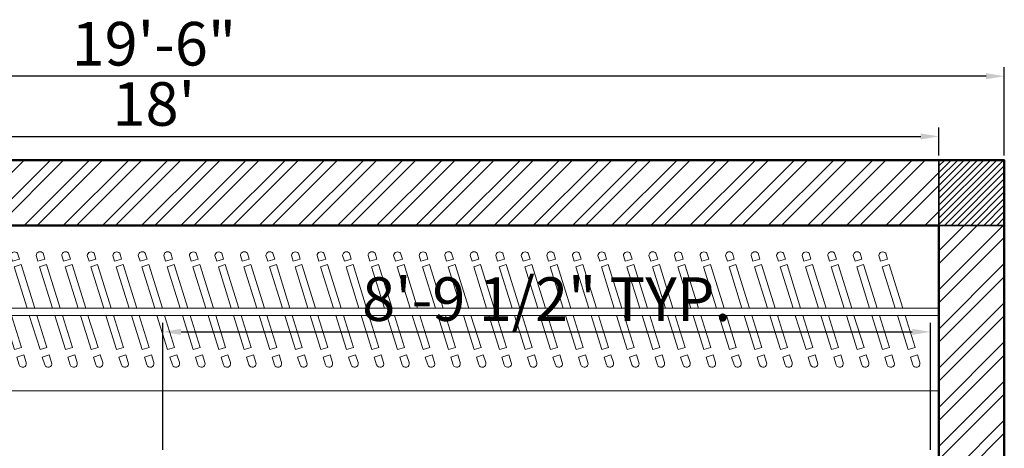
# Model space of a CAD drawing. Units: millimetres. Extents: x 20768 to 23556, y 50760 to 52704.
# Tile 23 of 36: x 20998 to 21133, y 52483 to 52542. Entities that reach past the tile are written whole.
import ezdxf

# ---------------------------------------------------------------- set-up
doc = ezdxf.new("R2010")
doc.units = ezdxf.units.MM
for name, color, linetype, lineweight in [('A-ANNO-DIMS', 2, 'Continuous', 18), ('A-FURN', 8, 'Continuous', 18), ('A-WALL', 7, 'Continuous', 50), ('A-WALL-PATT', 8, 'Continuous', 13), ('S-ANNO-DIMS', 2, 'Continuous', 18), ('S-COLS', 20, 'Continuous', 35)]:
    doc.layers.add(name, color=color, linetype=linetype, lineweight=lineweight)
doc.styles.get("Standard").update_dxf_attribs({"font": 'arial.ttf'})
doc.dimstyles.new('ISO-25', dxfattribs={"dimtxt": 6, "dimasz": 2.5, "dimexe": 1.25, "dimexo": 0.625, "dimtad": 1, "dimdec": 0, "dimlunit": 3, "dimtxsty": 'Standard', "dimcen": 2.5, "dimadec": 0, "dimazin": 0, "dimtfac": 1, "dimtdec": 0, "dimtmove": 0, "dimatfit": 3, "dimfxl": 1, "dimarcsym": 0})
pattern_1 = [(45, (-81.1113, 0), (-2.69407684, 2.69407684), []), (45, (-79.3152, 0), (-2.69407684, 2.69407684), [])]

# ---------------------------------------------------------------- blocks, each defined once
blk = doc.blocks.new('wb')
for p, q in [((21205.25, 52502.52), (21061.44, 52502.52)), ((21205.25, 52501.52), (21061.44, 52501.52))]:
    blk.add_line(p, q)
blk.add_lwpolyline([(21205.25, 52513.9), (21061.44, 52513.9), (21061.44, 52491.15), (21205.25, 52491.15)], close=True)
for points in [[(21064.45, 52510.07, 0.695903), (21063.5, 52509.77), (21063.75, 52508.98), (21064.7, 52509.27)], [(21067.97, 52510.07, 0.695903), (21067.01, 52509.77), (21067.26, 52508.98), (21068.21, 52509.27)], [(21071.48, 52510.07, 0.695903), (21070.52, 52509.77), (21070.77, 52508.98), (21071.73, 52509.27)], [(21074.99, 52510.07, 0.695903), (21074.04, 52509.77), (21074.28, 52508.98), (21075.24, 52509.27)], [(21078.5, 52510.07, 0.695903), (21077.55, 52509.77), (21077.8, 52508.98), (21078.75, 52509.27)], [(21082.02, 52510.07, 0.695903), (21081.06, 52509.77), (21081.31, 52508.98), (21082.26, 52509.27)], [(21085.53, 52510.07, 0.695903), (21084.57, 52509.77), (21084.82, 52508.98), (21085.78, 52509.27)], [(21089.04, 52510.07, 0.695903), (21088.09, 52509.77), (21088.33, 52508.98), (21089.29, 52509.27)], [(21092.55, 52510.07, 0.695903), (21091.6, 52509.77), (21091.85, 52508.98), (21092.8, 52509.27)], [(21096.07, 52510.07, 0.695903), (21095.11, 52509.77), (21095.36, 52508.98), (21096.31, 52509.27)], [(21099.58, 52510.07, 0.695903), (21098.62, 52509.77), (21098.87, 52508.98), (21099.83, 52509.27)], [(21103.09, 52510.07, 0.695903), (21102.14, 52509.77), (21102.38, 52508.98), (21103.34, 52509.27)], [(21106.6, 52510.07, 0.695903), (21105.65, 52509.77), (21105.9, 52508.98), (21106.85, 52509.27)], [(21110.12, 52510.07, 0.695903), (21109.16, 52509.77), (21109.41, 52508.98), (21110.36, 52509.27)], [(21113.63, 52510.07, 0.695903), (21112.67, 52509.77), (21112.92, 52508.98), (21113.88, 52509.27)], [(21117.14, 52510.07, 0.695903), (21116.19, 52509.77), (21116.43, 52508.98), (21117.39, 52509.27)], [(21120.65, 52510.07, 0.695903), (21119.7, 52509.77), (21119.95, 52508.98), (21120.9, 52509.27)], [(21124.17, 52510.07, 0.695903), (21123.21, 52509.77), (21123.46, 52508.98), (21124.41, 52509.27)], [(21127.68, 52510.07, 0.695903), (21126.72, 52509.77), (21126.97, 52508.98), (21127.93, 52509.27)], [(21131.19, 52510.07, 0.695903), (21130.24, 52509.77), (21130.48, 52508.98), (21131.44, 52509.27)], [(21134.7, 52510.07, 0.695903), (21133.75, 52509.77), (21134, 52508.98), (21134.95, 52509.27)], [(21138.22, 52510.07, 0.695903), (21137.26, 52509.77), (21137.51, 52508.98), (21138.46, 52509.27)], [(21141.73, 52510.07, 0.695903), (21140.77, 52509.77), (21141.02, 52508.98), (21141.98, 52509.27)], [(21145.24, 52510.07, 0.695903), (21144.29, 52509.77), (21144.54, 52508.98), (21145.49, 52509.27)], [(21148.75, 52510.07, 0.695903), (21147.8, 52509.77), (21148.05, 52508.98), (21149, 52509.27)], [(21152.27, 52510.07, 0.695903), (21151.31, 52509.77), (21151.56, 52508.98), (21152.52, 52509.27)], [(21155.78, 52510.07, 0.695903), (21154.83, 52509.77), (21155.07, 52508.98), (21156.03, 52509.27)], [(21159.29, 52510.07, 0.695903), (21158.34, 52509.77), (21158.59, 52508.98), (21159.54, 52509.27)], [(21162.8, 52510.07, 0.695903), (21161.85, 52509.77), (21162.1, 52508.98), (21163.05, 52509.27)], [(21166.32, 52510.07, 0.695903), (21165.36, 52509.77), (21165.61, 52508.98), (21166.57, 52509.27)], [(21169.83, 52510.07, 0.695903), (21168.88, 52509.77), (21169.12, 52508.98), (21170.08, 52509.27)], [(21173.34, 52510.07, 0.695903), (21172.39, 52509.77), (21172.64, 52508.98), (21173.59, 52509.27)], [(21176.86, 52510.07, 0.695903), (21175.9, 52509.77), (21176.15, 52508.98), (21177.1, 52509.27)], [(21180.37, 52510.07, 0.695903), (21179.41, 52509.77), (21179.66, 52508.98), (21180.62, 52509.27)], [(21183.88, 52510.07, 0.695903), (21182.93, 52509.77), (21183.17, 52508.98), (21184.13, 52509.27)], [(21187.39, 52510.07, 0.695903), (21186.44, 52509.77), (21186.69, 52508.98), (21187.64, 52509.27)], [(21190.91, 52510.07, 0.695903), (21189.95, 52509.77), (21190.2, 52508.98), (21191.15, 52509.27)], [(21194.42, 52510.07, 0.695903), (21193.46, 52509.77), (21193.71, 52508.98), (21194.67, 52509.27)], [(21197.93, 52510.07, 0.695903), (21196.98, 52509.77), (21197.22, 52508.98), (21198.18, 52509.27)], [(21068.81, 52496.1), (21067.85, 52495.8), (21068.19, 52494.73, 1), (21069.14, 52495.03)], [(21072.32, 52496.1), (21071.37, 52495.8), (21071.7, 52494.73, 1), (21072.65, 52495.03)], [(21075.83, 52496.1), (21074.88, 52495.8), (21075.21, 52494.73, 1), (21076.17, 52495.03)], [(21079.35, 52496.1), (21078.39, 52495.8), (21078.73, 52494.73, 1), (21079.68, 52495.03)], [(21082.86, 52496.1), (21081.9, 52495.8), (21082.24, 52494.73, 1), (21083.19, 52495.03)], [(21086.37, 52496.1), (21085.42, 52495.8), (21085.75, 52494.73, 1), (21086.7, 52495.03)], [(21089.88, 52496.1), (21088.93, 52495.8), (21089.26, 52494.73, 1), (21090.22, 52495.03)], [(21093.4, 52496.1), (21092.44, 52495.8), (21092.78, 52494.73, 1), (21093.73, 52495.03)], [(21096.91, 52496.1), (21095.95, 52495.8), (21096.29, 52494.73, 1), (21097.24, 52495.03)], [(21100.42, 52496.1), (21099.47, 52495.8), (21099.8, 52494.73, 1), (21100.76, 52495.03)], [(21103.93, 52496.1), (21102.98, 52495.8), (21103.31, 52494.73, 1), (21104.27, 52495.03)], [(21107.45, 52496.1), (21106.49, 52495.8), (21106.83, 52494.73, 1), (21107.78, 52495.03)], [(21110.96, 52496.1), (21110, 52495.8), (21110.34, 52494.73, 1), (21111.29, 52495.03)], [(21114.47, 52496.1), (21113.52, 52495.8), (21113.85, 52494.73, 1), (21114.81, 52495.03)], [(21117.98, 52496.1), (21117.03, 52495.8), (21117.36, 52494.73, 1), (21118.32, 52495.03)], [(21121.5, 52496.1), (21120.54, 52495.8), (21120.88, 52494.73, 1), (21121.83, 52495.03)], [(21125.01, 52496.1), (21124.05, 52495.8), (21124.39, 52494.73, 1), (21125.34, 52495.03)], [(21128.52, 52496.1), (21127.57, 52495.8), (21127.9, 52494.73, 1), (21128.86, 52495.03)], [(21132.03, 52496.1), (21131.08, 52495.8), (21131.41, 52494.73, 1), (21132.37, 52495.03)], [(21135.55, 52496.1), (21134.59, 52495.8), (21134.93, 52494.73, 1), (21135.88, 52495.03)], [(21139.06, 52496.1), (21138.1, 52495.8), (21138.44, 52494.73, 1), (21139.39, 52495.03)], [(21142.57, 52496.1), (21141.62, 52495.8), (21141.95, 52494.73, 1), (21142.91, 52495.03)], [(21146.08, 52496.1), (21145.13, 52495.8), (21145.46, 52494.73, 1), (21146.42, 52495.03)], [(21149.6, 52496.1), (21148.64, 52495.8), (21148.98, 52494.73, 1), (21149.93, 52495.03)], [(21153.11, 52496.1), (21152.15, 52495.8), (21152.49, 52494.73, 1), (21153.44, 52495.03)], [(21156.62, 52496.1), (21155.67, 52495.8), (21156, 52494.73, 1), (21156.96, 52495.03)], [(21160.13, 52496.1), (21159.18, 52495.8), (21159.51, 52494.73, 1), (21160.47, 52495.03)], [(21163.65, 52496.1), (21162.69, 52495.8), (21163.03, 52494.73, 1), (21163.98, 52495.03)], [(21167.16, 52496.1), (21166.2, 52495.8), (21166.54, 52494.73, 1), (21167.49, 52495.03)], [(21170.67, 52496.1), (21169.72, 52495.8), (21170.05, 52494.73, 1), (21171.01, 52495.03)], [(21174.18, 52496.1), (21173.23, 52495.8), (21173.56, 52494.73, 1), (21174.52, 52495.03)], [(21177.7, 52496.1), (21176.74, 52495.8), (21177.08, 52494.73, 1), (21178.03, 52495.03)], [(21181.21, 52496.1), (21180.25, 52495.8), (21180.59, 52494.73, 1), (21181.54, 52495.03)], [(21184.72, 52496.1), (21183.77, 52495.8), (21184.1, 52494.73, 1), (21185.06, 52495.03)], [(21188.23, 52496.1), (21187.28, 52495.8), (21187.61, 52494.73, 1), (21188.57, 52495.03)], [(21191.75, 52496.1), (21190.79, 52495.8), (21191.13, 52494.73, 1), (21192.08, 52495.03)], [(21195.26, 52496.1), (21194.31, 52495.8), (21194.64, 52494.73, 1), (21195.59, 52495.03)], [(21198.77, 52496.1), (21197.82, 52495.8), (21198.15, 52494.73, 1), (21199.11, 52495.03)], [(21202.29, 52496.1), (21201.33, 52495.8), (21201.67, 52494.73, 1), (21202.62, 52495.03)]]:
    blk.add_lwpolyline(points, format="xyb", close=True)
for points in [[(21065.76, 52502.52), (21063.98, 52508.23), (21064.93, 52508.53), (21066.81, 52502.52)], [(21069.27, 52502.52), (21067.49, 52508.23), (21068.44, 52508.53), (21070.32, 52502.52)], [(21072.78, 52502.52), (21071, 52508.23), (21071.96, 52508.53), (21073.83, 52502.52)], [(21076.3, 52502.52), (21074.51, 52508.23), (21075.47, 52508.53), (21077.34, 52502.52)], [(21079.81, 52502.52), (21078.03, 52508.23), (21078.98, 52508.53), (21080.86, 52502.52)], [(21083.32, 52502.52), (21081.54, 52508.23), (21082.49, 52508.53), (21084.37, 52502.52)], [(21086.83, 52502.52), (21085.05, 52508.23), (21086.01, 52508.53), (21087.88, 52502.52)], [(21090.35, 52502.52), (21088.57, 52508.23), (21089.52, 52508.53), (21091.39, 52502.52)], [(21093.86, 52502.52), (21092.08, 52508.23), (21093.03, 52508.53), (21094.91, 52502.52)], [(21097.37, 52502.52), (21095.59, 52508.23), (21096.55, 52508.53), (21098.42, 52502.52)], [(21100.88, 52502.52), (21099.1, 52508.23), (21100.06, 52508.53), (21101.93, 52502.52)], [(21104.4, 52502.52), (21102.62, 52508.23), (21103.57, 52508.53), (21105.44, 52502.52)], [(21107.91, 52502.52), (21106.13, 52508.23), (21107.08, 52508.53), (21108.96, 52502.52)], [(21111.42, 52502.52), (21109.64, 52508.23), (21110.6, 52508.53), (21112.47, 52502.52)], [(21114.93, 52502.52), (21113.15, 52508.23), (21114.11, 52508.53), (21115.98, 52502.52)], [(21118.45, 52502.52), (21116.67, 52508.23), (21117.62, 52508.53), (21119.49, 52502.52)], [(21121.96, 52502.52), (21120.18, 52508.23), (21121.13, 52508.53), (21123.01, 52502.52)], [(21125.47, 52502.52), (21123.69, 52508.23), (21124.65, 52508.53), (21126.52, 52502.52)], [(21128.98, 52502.52), (21127.2, 52508.23), (21128.16, 52508.53), (21130.03, 52502.52)], [(21132.5, 52502.52), (21130.72, 52508.23), (21131.67, 52508.53), (21133.54, 52502.52)], [(21136.01, 52502.52), (21134.23, 52508.23), (21135.18, 52508.53), (21137.06, 52502.52)], [(21139.52, 52502.52), (21137.74, 52508.23), (21138.7, 52508.53), (21140.57, 52502.52)], [(21143.03, 52502.52), (21141.25, 52508.23), (21142.21, 52508.53), (21144.08, 52502.52)], [(21146.55, 52502.52), (21144.77, 52508.23), (21145.72, 52508.53), (21147.59, 52502.52)], [(21150.06, 52502.52), (21148.28, 52508.23), (21149.23, 52508.53), (21151.11, 52502.52)], [(21153.57, 52502.52), (21151.79, 52508.23), (21152.75, 52508.53), (21154.62, 52502.52)], [(21157.08, 52502.52), (21155.3, 52508.23), (21156.26, 52508.53), (21158.13, 52502.52)], [(21160.6, 52502.52), (21158.82, 52508.23), (21159.77, 52508.53), (21161.64, 52502.52)], [(21164.11, 52502.52), (21162.33, 52508.23), (21163.28, 52508.53), (21165.16, 52502.52)], [(21167.62, 52502.52), (21165.84, 52508.23), (21166.8, 52508.53), (21168.67, 52502.52)], [(21171.13, 52502.52), (21169.35, 52508.23), (21170.31, 52508.53), (21172.18, 52502.52)], [(21174.65, 52502.52), (21172.87, 52508.23), (21173.82, 52508.53), (21175.69, 52502.52)], [(21178.16, 52502.52), (21176.38, 52508.23), (21177.33, 52508.53), (21179.21, 52502.52)], [(21181.67, 52502.52), (21179.89, 52508.23), (21180.85, 52508.53), (21182.72, 52502.52)], [(21185.19, 52502.52), (21183.4, 52508.23), (21184.36, 52508.53), (21186.23, 52502.52)], [(21188.7, 52502.52), (21186.92, 52508.23), (21187.87, 52508.53), (21189.75, 52502.52)], [(21192.21, 52502.52), (21190.43, 52508.23), (21191.38, 52508.53), (21193.26, 52502.52)], [(21195.72, 52502.52), (21193.94, 52508.23), (21194.9, 52508.53), (21196.77, 52502.52)], [(21199.24, 52502.52), (21197.46, 52508.23), (21198.41, 52508.53), (21200.28, 52502.52)], [(21066.07, 52501.52), (21067.54, 52496.81), (21068.49, 52497.1), (21067.12, 52501.52)], [(21069.58, 52501.52), (21071.05, 52496.81), (21072.01, 52497.1), (21070.63, 52501.52)], [(21073.09, 52501.52), (21074.57, 52496.81), (21075.52, 52497.1), (21074.14, 52501.52)], [(21076.61, 52501.52), (21078.08, 52496.81), (21079.03, 52497.1), (21077.65, 52501.52)], [(21080.12, 52501.52), (21081.59, 52496.81), (21082.55, 52497.1), (21081.17, 52501.52)], [(21083.63, 52501.52), (21085.1, 52496.81), (21086.06, 52497.1), (21084.68, 52501.52)], [(21087.14, 52501.52), (21088.62, 52496.81), (21089.57, 52497.1), (21088.19, 52501.52)], [(21090.66, 52501.52), (21092.13, 52496.81), (21093.08, 52497.1), (21091.7, 52501.52)], [(21094.17, 52501.52), (21095.64, 52496.81), (21096.6, 52497.1), (21095.22, 52501.52)], [(21097.68, 52501.52), (21099.15, 52496.81), (21100.11, 52497.1), (21098.73, 52501.52)], [(21101.2, 52501.52), (21102.67, 52496.81), (21103.62, 52497.1), (21102.24, 52501.52)], [(21104.71, 52501.52), (21106.18, 52496.81), (21107.13, 52497.1), (21105.76, 52501.52)], [(21108.22, 52501.52), (21109.69, 52496.81), (21110.65, 52497.1), (21109.27, 52501.52)], [(21111.73, 52501.52), (21113.2, 52496.81), (21114.16, 52497.1), (21112.78, 52501.52)], [(21115.25, 52501.52), (21116.72, 52496.81), (21117.67, 52497.1), (21116.29, 52501.52)], [(21118.76, 52501.52), (21120.23, 52496.81), (21121.18, 52497.1), (21119.81, 52501.52)], [(21122.27, 52501.52), (21123.74, 52496.81), (21124.7, 52497.1), (21123.32, 52501.52)], [(21125.78, 52501.52), (21127.25, 52496.81), (21128.21, 52497.1), (21126.83, 52501.52)], [(21129.3, 52501.52), (21130.77, 52496.81), (21131.72, 52497.1), (21130.34, 52501.52)], [(21132.81, 52501.52), (21134.28, 52496.81), (21135.23, 52497.1), (21133.86, 52501.52)], [(21136.32, 52501.52), (21137.79, 52496.81), (21138.75, 52497.1), (21137.37, 52501.52)], [(21139.83, 52501.52), (21141.3, 52496.81), (21142.26, 52497.1), (21140.88, 52501.52)], [(21143.35, 52501.52), (21144.82, 52496.81), (21145.77, 52497.1), (21144.39, 52501.52)], [(21146.86, 52501.52), (21148.33, 52496.81), (21149.28, 52497.1), (21147.91, 52501.52)], [(21150.37, 52501.52), (21151.84, 52496.81), (21152.8, 52497.1), (21151.42, 52501.52)], [(21153.88, 52501.52), (21155.35, 52496.81), (21156.31, 52497.1), (21154.93, 52501.52)], [(21157.4, 52501.52), (21158.87, 52496.81), (21159.82, 52497.1), (21158.44, 52501.52)], [(21160.91, 52501.52), (21162.38, 52496.81), (21163.33, 52497.1), (21161.96, 52501.52)], [(21164.42, 52501.52), (21165.89, 52496.81), (21166.85, 52497.1), (21165.47, 52501.52)], [(21167.93, 52501.52), (21169.4, 52496.81), (21170.36, 52497.1), (21168.98, 52501.52)], [(21171.45, 52501.52), (21172.92, 52496.81), (21173.87, 52497.1), (21172.49, 52501.52)], [(21174.96, 52501.52), (21176.43, 52496.81), (21177.38, 52497.1), (21176.01, 52501.52)], [(21178.47, 52501.52), (21179.94, 52496.81), (21180.9, 52497.1), (21179.52, 52501.52)], [(21181.98, 52501.52), (21183.46, 52496.81), (21184.41, 52497.1), (21183.03, 52501.52)], [(21185.5, 52501.52), (21186.97, 52496.81), (21187.92, 52497.1), (21186.54, 52501.52)], [(21189.01, 52501.52), (21190.48, 52496.81), (21191.43, 52497.1), (21190.06, 52501.52)], [(21192.52, 52501.52), (21193.99, 52496.81), (21194.95, 52497.1), (21193.57, 52501.52)], [(21196.03, 52501.52), (21197.51, 52496.81), (21198.46, 52497.1), (21197.08, 52501.52)], [(21199.55, 52501.52), (21201.02, 52496.81), (21201.97, 52497.1), (21200.59, 52501.52)]]:
    blk.add_lwpolyline(points)
blk = doc.blocks.new('*D109')
at = {"layer": 'A-ANNO-DIMS', "color": 0, "lineweight": -2, "transparency": 16777216}
for p, q in [((20899.14, 52523.52), (20899.14, 52535.7)), ((21133.14, 52523.52), (21133.14, 52535.7)), ((21130.64, 52534.45), (20901.64, 52534.45))]:
    blk.add_line(p, q, dxfattribs=at)
at = {"layer": 'A-ANNO-DIMS', "color": 0, "transparency": 16777216}
for points in [[(20901.64, 52534.87), (20901.64, 52534.03), (20899.14, 52534.45)], [(21130.64, 52534.87), (21130.64, 52534.03), (21133.14, 52534.45)]]:
    blk.add_solid(points, dxfattribs=at)
at = {"layer": 'Defpoints', "color": 0, "transparency": 16777216}
for p in [(20899.14, 52534.45), (20899.14, 52522.9), (21133.14, 52522.9)]:
    blk.add_point(p, dxfattribs=at)
at = {"layer": 'A-ANNO-DIMS', "color": 0, "transparency": 16777216, "insert": (21016.14, 52538.14), "char_height": 6, "attachment_point": 5}
blk.add_mtext('19\'-6"', dxfattribs=at)
blk = doc.blocks.new('*D110')
at = {"layer": 'A-ANNO-DIMS', "color": 0, "lineweight": -2, "transparency": 16777216}
for p, q in [((20908.14, 52523.52), (20908.14, 52527.41)), ((21124.14, 52523.52), (21124.14, 52527.41)), ((20910.64, 52526.16), (21121.64, 52526.16))]:
    blk.add_line(p, q, dxfattribs=at)
at = {"layer": 'A-ANNO-DIMS', "color": 0, "transparency": 16777216}
for points in [[(20910.64, 52526.57), (20910.64, 52525.74), (20908.14, 52526.16)], [(21121.64, 52526.57), (21121.64, 52525.74), (21124.14, 52526.16)]]:
    blk.add_solid(points, dxfattribs=at)
at = {"layer": 'Defpoints', "color": 0, "transparency": 16777216}
for p in [(21124.14, 52526.16), (20908.14, 52522.9), (21124.14, 52522.9)]:
    blk.add_point(p, dxfattribs=at)
at = {"layer": 'A-ANNO-DIMS', "color": 0, "transparency": 16777216, "insert": (21016.14, 52529.85), "char_height": 6, "attachment_point": 5}
blk.add_mtext("18'", dxfattribs=at)
blk = doc.blocks.new('*D190')
at = {"layer": 'Defpoints', "color": 0, "transparency": 16777216}
for p in [(21122.97, 52499.26), (21017.38, 52482.4), (21122.97, 52482.4)]:
    blk.add_point(p, dxfattribs=at)
at = {"layer": 'S-ANNO-DIMS', "color": 0, "lineweight": -2, "transparency": 16777216}
for p, q in [((21017.38, 52483.02), (21017.38, 52500.51)), ((21122.97, 52483.02), (21122.97, 52500.51)), ((21019.88, 52499.26), (21120.47, 52499.26))]:
    blk.add_line(p, q, dxfattribs=at)
at = {"layer": 'S-ANNO-DIMS', "color": 0, "transparency": 16777216}
for points in [[(21019.88, 52499.68), (21019.88, 52498.84), (21017.38, 52499.26)], [(21120.47, 52499.68), (21120.47, 52498.84), (21122.97, 52499.26)]]:
    blk.add_solid(points, dxfattribs=at)
at = {"layer": 'S-ANNO-DIMS', "color": 0, "transparency": 16777216, "insert": (21070.17, 52502.99), "char_height": 6, "attachment_point": 5}
blk.add_mtext('8\'-9 1/2" TYP.', dxfattribs=at)

msp = doc.modelspace()

# ---------------------------------------------------------------- hatches: boundary and pattern name
at = {"layer": 'A-WALL-PATT'}
h = msp.add_hatch(dxfattribs=at)
h.set_pattern_fill('ANSI32', color=256, scale=0.4)
h.set_pattern_definition(pattern_1)
h.paths.add_polyline_path([(21124.14, 52522.9), (20908.14, 52522.9), (20908.14, 52513.9), (21124.14, 52513.9)])
h = msp.add_hatch(dxfattribs=at)
h.set_pattern_fill('ANSI31', color=256, scale=0.2)
h.set_pattern_definition([(45, (-81.11126, 0), (-0.449012806, 0.449012806), [])])
h.paths.add_polyline_path([(21133.14, 52522.9), (21124.14, 52522.9), (21124.14, 52513.9), (21133.14, 52513.9)])
h = msp.add_hatch(dxfattribs=at)
h.set_pattern_fill('ANSI32', color=256, scale=0.4)
h.set_pattern_definition(pattern_1)
h.paths.add_polyline_path([(21133.14, 52513.9), (21124.14, 52513.9), (21124.14, 52335.9), (21133.14, 52335.9)])

# ---------------------------------------------------------------- linework, layer by layer
at = {"layer": 'A-WALL'}
for p, q in [((20899.14, 52522.9), (21133.14, 52522.9)), ((21133.14, 52522.9), (21133.14, 51829.9)), ((20908.14, 52513.9), (21124.14, 52513.9)), ((21124.14, 52513.9), (21124.14, 51838.9))]:
    msp.add_line(p, q, dxfattribs=at)
at = {"layer": 'S-COLS'}
msp.add_lwpolyline([(21124.14, 52513.9), (21133.14, 52513.9), (21133.14, 52522.9), (21124.14, 52522.9)], close=True, dxfattribs=at)

# ---------------------------------------------------------------- block references
at = {"layer": 'A-FURN'}
msp.add_blockref('wb', (-81.11, 0), dxfattribs=at)

# ---------------------------------------------------------------- dimensions: what is measured, and where the dimension line sits
at = {"layer": 'A-ANNO-DIMS'}
for base, p1, p2, picture, middle in [((20899.14, 52534.45), (21133.14, 52522.9), (20899.14, 52522.9), '*D109', (21016.14, 52538.14)), ((21124.14, 52526.16), (20908.14, 52522.9), (21124.14, 52522.9), '*D110', (21016.14, 52529.85))]:
    dim = msp.add_linear_dim(base=base, p1=p1, p2=p2, dimstyle='ISO-25', override={"dimclrd": 0, "dimclre": 0, "dimclrt": 0}, dxfattribs=at)
    dim.commit()
    dim.dimension.update_dxf_attribs({"geometry": picture, "text_midpoint": middle})
at = {"layer": 'S-ANNO-DIMS'}
dim = msp.add_linear_dim(base=(21122.97, 52499.26), p1=(21017.38, 52482.4), p2=(21122.97, 52482.4), text='<> TYP.', dimstyle='ISO-25', override={"dimdec": 1, "dimrnd": 0, "dimzin": 1, "dimlunit": 4, "dimfrac": 2}, dxfattribs=at)
dim.commit()
dim.dimension.update_dxf_attribs({"geometry": '*D190', "text_midpoint": (21070.17, 52502.99)})

doc.saveas('drawing.dxf')
